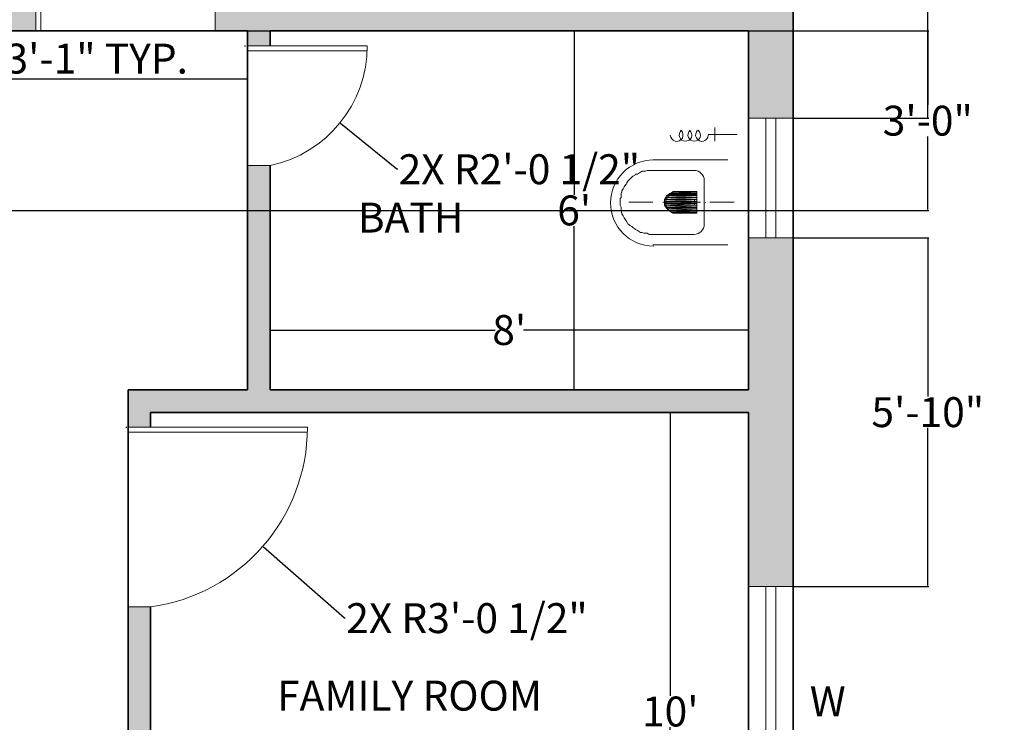
# Model space of a CAD drawing. Units: inches. Extents: x 302 to 1258, y 831 to 1373.
# Tile 5 of 13: x 569 to 767, y 1070 to 1211. Entities that reach past the tile are written whole.
import ezdxf

# ---------------------------------------------------------------- set-up
doc = ezdxf.new("R2010")
doc.units = ezdxf.units.IN
doc.header["$MEASUREMENT"] = 0
for name, color, linetype, lineweight in [('A-ANNO-DIMS', 2, 'Continuous', 18), ('A-ANNO-TEXT', 7, 'Continuous', 18), ('A-AREA-IDEN', 7, 'Continuous', 18), ('A-DOOR', 3, 'Continuous', 18), ('A-FLOR-FIXT', 8, 'Continuous', 18), ('A-GLAZ', 4, 'Continuous', 18), ('A-WALL', 7, 'Continuous', 35), ('A-WALL-PATT', 251, 'Continuous', 13)]:
    doc.layers.add(name, color=color, linetype=linetype, lineweight=lineweight)
doc.styles.get("Standard").update_dxf_attribs({"font": 'arial.ttf'})
doc.dimstyles.get("Standard").update_dxf_attribs({"dimtxt": 6, "dimasz": 0.18, "dimexe": 0.18, "dimexo": 0.0625, "dimgap": 0.09, "dimtad": 0, "dimtih": 1, "dimtoh": 1, "dimdec": 1, "dimzin": 0, "dimdsep": 46, "dimlunit": 3, "dimtxsty": 'Standard', "dimcen": 0.09, "dimadec": 0, "dimazin": 0, "dimtfac": 1, "dimtdec": 1, "dimtofl": 0, "dimtmove": 0, "dimatfit": 3, "dimfxl": 1, "dimtolj": 1, "dimtzin": 0, "dimarcsym": 0})

# ---------------------------------------------------------------- blocks, each defined once
blk = doc.blocks.new('*D9')
at = {"layer": 'A-ANNO-DIMS', "color": 0, "lineweight": -2, "transparency": 16777216}
for p, q in [((619.67, 1136.88), (619.67, 1149.01)), ((619.85, 1148.83), (664.82, 1148.83)), ((715.49, 1148.83), (670.52, 1148.83)), ((715.67, 1136.88), (715.67, 1149.01))]:
    blk.add_line(p, q, dxfattribs=at)
at = {"layer": 'A-ANNO-DIMS', "color": 0, "transparency": 16777216}
for points in [[(619.85, 1148.86), (619.85, 1148.8), (619.67, 1148.83)], [(715.49, 1148.86), (715.49, 1148.8), (715.67, 1148.83)]]:
    blk.add_solid(points, dxfattribs=at)
at = {"layer": 'Defpoints', "color": 0, "transparency": 16777216}
for p in [(715.67, 1148.83), (619.67, 1136.82), (715.67, 1136.82)]:
    blk.add_point(p, dxfattribs=at)
at = {"layer": 'A-ANNO-DIMS', "color": 0, "transparency": 16777216, "insert": (667.67, 1148.83), "char_height": 6, "attachment_point": 5}
blk.add_mtext("\\A1;8'", dxfattribs=at)
blk = doc.blocks.new('*D10')
at = {"layer": 'A-ANNO-DIMS', "color": 0, "lineweight": -2, "transparency": 16777216}
for p, q in [((715.61, 1208.82), (680.52, 1208.82)), ((680.7, 1208.64), (680.7, 1175.97)), ((680.7, 1137), (680.7, 1169.67)), ((715.61, 1136.82), (680.52, 1136.82))]:
    blk.add_line(p, q, dxfattribs=at)
at = {"layer": 'A-ANNO-DIMS', "color": 0, "transparency": 16777216}
for points in [[(680.67, 1208.64), (680.73, 1208.64), (680.7, 1208.82)], [(680.67, 1137), (680.73, 1137), (680.7, 1136.82)]]:
    blk.add_solid(points, dxfattribs=at)
at = {"layer": 'Defpoints', "color": 0, "transparency": 16777216}
for p in [(715.67, 1208.82), (680.7, 1136.82), (715.67, 1136.82)]:
    blk.add_point(p, dxfattribs=at)
at = {"layer": 'A-ANNO-DIMS', "color": 0, "transparency": 16777216, "insert": (680.7, 1172.82), "char_height": 6, "attachment_point": 5}
blk.add_mtext("\\A1;6'", dxfattribs=at)
blk = doc.blocks.new('*D12')
at = {"layer": 'A-ANNO-DIMS', "color": 0, "lineweight": -2, "transparency": 16777216}
for p, q in [((715.61, 1132.32), (699.81, 1132.32)), ((699.99, 1132.14), (699.99, 1075.47)), ((699.99, 1012.5), (699.99, 1069.17)), ((715.61, 1012.32), (699.81, 1012.32))]:
    blk.add_line(p, q, dxfattribs=at)
at = {"layer": 'A-ANNO-DIMS', "color": 0, "transparency": 16777216}
for points in [[(699.96, 1132.14), (700.02, 1132.14), (699.99, 1132.32)], [(699.96, 1012.5), (700.02, 1012.5), (699.99, 1012.32)]]:
    blk.add_solid(points, dxfattribs=at)
at = {"layer": 'Defpoints', "color": 0, "transparency": 16777216}
for p in [(715.67, 1132.32), (699.99, 1012.32), (715.67, 1012.32)]:
    blk.add_point(p, dxfattribs=at)
at = {"layer": 'A-ANNO-DIMS', "color": 0, "transparency": 16777216, "insert": (699.99, 1072.32), "char_height": 6, "attachment_point": 5}
blk.add_mtext("\\A1;10'", dxfattribs=at)
blk = doc.blocks.new('*D16')
at = {"layer": 'A-ANNO-DIMS', "color": 0, "lineweight": -2, "transparency": 16777216}
for p, q in [((459.17, 1208.76), (459.17, 1198.98)), ((615.17, 1208.76), (615.17, 1198.98)), ((459.35, 1199.16), (532.27, 1199.16)), ((614.99, 1199.16), (542.07, 1199.16))]:
    blk.add_line(p, q, dxfattribs=at)
at = {"layer": 'A-ANNO-DIMS', "color": 0, "transparency": 16777216}
for points in [[(459.35, 1199.19), (459.35, 1199.13), (459.17, 1199.16)], [(614.99, 1199.19), (614.99, 1199.13), (615.17, 1199.16)]]:
    blk.add_solid(points, dxfattribs=at)
at = {"layer": 'Defpoints', "color": 0, "transparency": 16777216}
for p in [(459.17, 1208.82), (615.17, 1208.82), (615.17, 1199.16)]:
    blk.add_point(p, dxfattribs=at)
at = {"layer": 'A-ANNO-DIMS', "color": 0, "transparency": 16777216, "insert": (537.17, 1199.16), "char_height": 6, "attachment_point": 5}
blk.add_mtext("\\A1;13'", dxfattribs=at)
blk = doc.blocks.new('WC-PLAN')
h = blk.add_hatch(color=256)
h.paths.add_polyline_path([(17.3, 10.16), (11.23, 10.16), (17.3, 9.71)])
h.paths.add_polyline_path([(11.23, 10.16), (17.3, 9.71), (11.08, 9.71)])
h = blk.add_hatch(color=256)
h.paths.add_polyline_path([(17.3, 10.32), (11.61, 10.32), (17.3, 10.16)])
h.paths.add_polyline_path([(11.61, 10.32), (17.3, 10.16), (11.23, 10.16)])
h = blk.add_hatch(color=256)
h.paths.add_polyline_path([(17.3, 10.54), (11.83, 10.54), (17.3, 10.32)])
h.paths.add_polyline_path([(11.83, 10.54), (17.3, 10.32), (11.61, 10.32)])
h = blk.add_hatch(color=256)
h.paths.add_polyline_path([(17.3, 10.7), (12.21, 10.7), (17.3, 10.54)])
h.paths.add_polyline_path([(12.21, 10.7), (17.3, 10.54), (11.83, 10.54)])
h = blk.add_hatch(color=256)
h.paths.add_polyline_path([(17.3, 10.92), (12.59, 10.92), (17.3, 10.7)])
h.paths.add_polyline_path([(12.59, 10.92), (17.3, 10.7), (12.21, 10.7)])
h = blk.add_hatch(color=256)
h.paths.add_polyline_path([(17.3, 9.71), (11.08, 9.71), (17.3, 9.33)])
h.paths.add_polyline_path([(11.08, 9.71), (17.3, 9.33), (10.85, 9.33)])
h = blk.add_hatch(color=256)
h.paths.add_polyline_path([(17.3, 9.33), (10.85, 9.33), (17.3, 8.95)])
h.paths.add_polyline_path([(10.85, 9.33), (17.3, 8.95), (10.85, 8.95)])
h = blk.add_hatch(color=256)
h.paths.add_polyline_path([(17.3, 8.95), (10.85, 8.95), (17.3, 8.57)])
h.paths.add_polyline_path([(10.85, 8.95), (17.3, 8.57), (10.85, 8.57)])
h = blk.add_hatch(color=256)
h.paths.add_polyline_path([(17.3, 8.57), (10.85, 8.57), (17.3, 8.19)])
h.paths.add_polyline_path([(10.85, 8.57), (17.3, 8.19), (10.85, 8.19)])
h = blk.add_hatch(color=256)
h.paths.add_polyline_path([(17.3, 8.19), (10.85, 8.19), (17.3, 7.81)])
h.paths.add_polyline_path([(10.85, 8.19), (17.3, 7.81), (11.08, 7.81)])
h = blk.add_hatch(color=256)
h.paths.add_polyline_path([(17.3, 7.81), (11.08, 7.81), (17.3, 7.59)])
h.paths.add_polyline_path([(11.08, 7.81), (17.3, 7.59), (11.23, 7.59)])
h = blk.add_hatch(color=256)
h.paths.add_polyline_path([(17.3, 7.59), (11.23, 7.59), (17.3, 7.21)])
h.paths.add_polyline_path([(11.23, 7.59), (17.3, 7.21), (11.61, 7.21)])
h = blk.add_hatch(color=256)
h.paths.add_polyline_path([(17.3, 7.21), (11.61, 7.21), (17.3, 7.05)])
h.paths.add_polyline_path([(11.61, 7.21), (17.3, 7.05), (11.83, 7.05)])
h = blk.add_hatch(color=256)
h.paths.add_polyline_path([(17.3, 7.05), (11.83, 7.05), (17.3, 6.83)])
h.paths.add_polyline_path([(11.83, 7.05), (17.3, 6.83), (12.21, 6.83)])
h = blk.add_hatch(color=256)
h.paths.add_polyline_path([(17.3, 6.83), (12.21, 6.83), (17.3, 6.6)])
h.paths.add_polyline_path([(12.21, 6.83), (17.3, 6.6), (12.59, 6.6)])
h.paths.add_polyline_path([(17.3, 6.6), (12.59, 6.6), (12.97, 6.6)])
for points in [[(20.94, 21.03), (20.94, 23.77), (20.94, 23.77)], [(25.41, 22.4), (19.57, 22.4), (19.57, 22.4)], [(23.52, 17.3), (8.5, 17.3), (8.5, 17.3)], [(9.48, 2.35), (8.72, 2.35), (8.12, 2.35), (7.74, 2.35), (7.36, 2.58), (6.98, 2.58), (6.75, 2.58), (6.37, 2.73), (5.99, 2.73), (5.61, 2.96), (5.39, 3.11), (5.01, 3.34), (4.85, 3.49), (4.48, 3.72), (4.25, 3.94), (3.87, 4.1), (3.64, 4.32), (3.49, 4.48), (3.26, 4.85), (3.11, 5.08), (2.88, 5.46), (2.73, 5.69), (2.5, 6.07), (2.28, 6.45), (2.28, 6.6), (2.12, 7.05), (2.12, 7.43), (2.12, 7.81), (1.9, 8.19), (1.9, 8.8), (1.9, 9.56), (2.12, 9.71), (2.12, 10.16), (2.12, 10.54), (2.28, 10.92), (2.28, 11.07), (2.5, 11.45), (2.73, 11.91), (2.88, 12.06), (3.11, 12.44), (3.26, 12.67), (3.49, 13.05), (3.64, 13.2), (3.87, 13.43), (4.25, 13.81), (4.48, 14.03), (4.85, 14.18), (5.01, 14.41), (5.39, 14.41), (5.61, 14.56), (5.99, 14.79), (6.37, 15.02), (6.75, 15.02), (6.98, 15.02), (7.36, 15.17), (7.74, 15.17), (8.12, 15.17), (8.72, 15.17), (9.48, 15.17)], [(16.69, 15.17), (9.48, 15.17), (9.48, 15.17)], [(18.81, 4.48), (18.81, 13.2), (18.81, 13.2)], [(17.3, 10.92), (12.97, 10.92), (12.97, 10.92)], [(17.3, 6.6), (17.3, 10.92), (17.3, 10.92)], [(8.5, 8.8), (3.64, 8.8), (3.64, 8.8)], [(18.05, 8.8), (10.47, 8.8), (10.47, 8.8)], [(16.84, 9.18), (16.92, 9.18), (16.92, 9.18)], [(16.84, 8.8), (16.84, 8.95), (16.84, 9.18)], [(16.84, 8.8), (16.92, 8.72), (16.92, 8.72)], [(16.84, 8.34), (16.84, 8.57), (16.84, 8.8)], [(16.84, 8.34), (16.92, 8.34), (16.92, 8.34)], [(19.04, 8.8), (19.04, 8.72), (19.04, 8.72)], [(24.81, 8.8), (19.95, 8.8), (19.95, 8.8)], [(17.3, 6.6), (12.97, 6.6), (12.97, 6.6)], [(16.69, 2.35), (9.48, 2.35), (9.48, 2.35)], [(23.52, 0.23), (8.5, 0.23), (8.5, 0.23)]]:
    blk.add_lwpolyline(points)
for points in [[(11.23, 10.16), (17.3, 9.71), (11.08, 9.71)], [(11.61, 10.32), (17.3, 10.16), (11.23, 10.16)], [(17.3, 10.16), (11.23, 10.16), (17.3, 9.71)], [(11.83, 10.54), (17.3, 10.32), (11.61, 10.32)], [(17.3, 10.32), (11.61, 10.32), (17.3, 10.16)], [(12.21, 10.7), (17.3, 10.54), (11.83, 10.54)], [(17.3, 10.54), (11.83, 10.54), (17.3, 10.32)], [(12.59, 10.92), (17.3, 10.7), (12.21, 10.7)], [(17.3, 10.7), (12.21, 10.7), (17.3, 10.54)], [(12.97, 10.92), (17.3, 10.92), (12.59, 10.92)], [(17.3, 10.92), (12.59, 10.92), (17.3, 10.7)], [(17.3, 10.92), (12.97, 10.92)], [(11.08, 9.71), (17.3, 9.33), (10.85, 9.33)], [(17.3, 9.33), (10.85, 9.33), (17.3, 8.95)], [(10.85, 9.33), (17.3, 8.95), (10.85, 8.95)], [(17.3, 8.95), (10.85, 8.95), (17.3, 8.57)], [(10.85, 8.95), (17.3, 8.57), (10.85, 8.57)], [(17.3, 8.57), (10.85, 8.57), (17.3, 8.19)], [(10.85, 8.57), (17.3, 8.19), (10.85, 8.19)], [(17.3, 8.19), (10.85, 8.19), (17.3, 7.81)], [(10.85, 8.19), (17.3, 7.81), (11.08, 7.81)], [(17.3, 9.71), (11.08, 9.71), (17.3, 9.33)], [(17.3, 7.81), (11.08, 7.81), (17.3, 7.59)], [(11.08, 7.81), (17.3, 7.59), (11.23, 7.59)], [(17.3, 7.59), (11.23, 7.59), (17.3, 7.21)], [(11.23, 7.59), (17.3, 7.21), (11.61, 7.21)], [(17.3, 7.21), (11.61, 7.21), (17.3, 7.05)], [(11.61, 7.21), (17.3, 7.05), (11.83, 7.05)], [(17.3, 7.05), (11.83, 7.05), (17.3, 6.83)], [(11.83, 7.05), (17.3, 6.83), (12.21, 6.83)], [(17.3, 6.83), (12.21, 6.83), (17.3, 6.6)], [(12.21, 6.83), (17.3, 6.6), (12.59, 6.6)], [(17.3, 6.6), (12.59, 6.6), (12.97, 6.6)], [(12.59, 6.6), (17.3, 6.6), (17.3, 6.6)]]:
    blk.add_lwpolyline(points, close=True)
for points, knots in [([(11.99, 22.25), (11.99, 21.72), (12.44, 21.19), (12.97, 21.03), (12.97, 21.03), (13.5, 20.88), (14.11, 21.19), (14.41, 21.64), (14.41, 21.64), (14.64, 22.17), (14.56, 22.78), (14.19, 23.16)], [0, 0, 0, 0, 0.083333, 0.083333, 0.083333, 0.083334, 0.166667, 0.166667, 0.166667, 0.166668, 1, 1, 1, 1]), ([(14.19, 23.23), (13.81, 22.86), (13.65, 22.32), (13.88, 21.79), (13.88, 21.79), (14.03, 21.34), (14.49, 21.03), (15.02, 21.03), (15.02, 21.03), (15.55, 21.03), (16.01, 21.34), (16.23, 21.79), (16.23, 21.79), (16.39, 22.32), (16.23, 22.86), (15.85, 23.23)], [0, 0, 0, 0, 0.0625, 0.0625, 0.0625, 0.062501, 0.125, 0.125, 0.125, 0.125001, 0.1875, 0.1875, 0.1875, 0.187501, 1, 1, 1, 1]), ([(15.93, 23.16), (15.55, 22.86), (15.4, 22.25), (15.63, 21.79), (15.63, 21.79), (15.78, 21.34), (16.31, 21.03), (16.76, 21.03), (16.76, 21.03), (17.3, 21.03), (17.75, 21.34), (17.98, 21.79), (17.98, 21.79), (18.13, 22.32), (17.98, 22.86), (17.6, 23.23)], [0, 0, 0, 0, 0.0625, 0.0625, 0.0625, 0.062501, 0.125, 0.125, 0.125, 0.125001, 0.1875, 0.1875, 0.1875, 0.187501, 1, 1, 1, 1]), ([(17.45, 23.23), (17.07, 22.86), (16.92, 22.17), (17.22, 21.72), (17.22, 21.72), (17.52, 21.19), (18.05, 20.88), (18.66, 21.03), (18.66, 21.03), (19.19, 21.19), (19.57, 21.72), (19.57, 22.25)], [0, 0, 0, 0, 0.083333, 0.083333, 0.083333, 0.083334, 0.166667, 0.166667, 0.166667, 0.166668, 1, 1, 1, 1]), ([(8.65, 17.3), (3.87, 17.3), (0, 13.43), (0, 8.65), (0, 8.65), (0, 3.87), (3.87, 0), (8.65, 0)], [0, 0, 0, 0, 0.125, 0.125, 0.125, 0.125001, 1, 1, 1, 1]), ([(13.12, 10.7), (11.99, 10.7), (11.08, 9.79), (11.08, 8.65), (11.08, 8.65), (11.08, 7.51), (11.99, 6.6), (13.12, 6.6)], [0, 0, 0, 0, 0.125, 0.125, 0.125, 0.125001, 1, 1, 1, 1])]:
    blk.add_open_spline(points, degree=3, knots=knots)
for points in [[(18.81, 13.12), (18.81, 14.26), (17.9, 15.17), (16.76, 15.17)], [(16.76, 2.35), (17.9, 2.35), (18.81, 3.26), (18.81, 4.4)]]:
    blk.add_open_spline(points, degree=3)
blk = doc.blocks.new('WINDOW-48IN')
for p, q in [((0, 0), (0, 9)), ((0, 9), (48, 9)), ((48, 9), (48, 0)), ((0, 5.5), (48, 5.5)), ((48, 3.5), (0, 3.5)), ((48, 0), (0, 0))]:
    blk.add_line(p, q)
blk = doc.blocks.new('VENT-WINDOW-24IN')
for p, q in [((0, 24), (9, 24)), ((0, 0), (0, 24)), ((3.5, 0), (3.5, 24)), ((5.5, 24), (5.5, 0)), ((9, 24), (9, 0)), ((9, 0), (0, 0))]:
    blk.add_line(p, q)
blk = doc.blocks.new('DOOR-36IN-BEDROOM')
for p, q in [((35, 36), (35, 0)), ((36, 0), (36, 36)), ((36, 36), (36, 0)), ((0, 0), (0, 4.5)), ((36, 0), (0, 0)), ((37, 0), (36, 0))]:
    blk.add_line(p, q)
blk.add_arc((36, -0.32), 36.32, 90, 172.3719)
blk = doc.blocks.new('DOOR-24IN-BATH')
for p, q in [((0, 27), (0, 24)), ((0, 24), (24, 24)), ((24, 24), (0, 24)), ((0, 24), (0, 0)), ((24, 23), (0, 23)), ((0, 0), (4.5, 0))]:
    blk.add_line(p, q)
blk.add_arc((-0.52, 24), 24.52, 281.8123, 0)
blk = doc.blocks.new('DOOR-36IN-ROOM')
for p, q in [((0, 39), (0, 36)), ((0, 36), (36, 36)), ((36, 36), (0, 36)), ((0, 36), (0, 0)), ((36, 35), (0, 35)), ((0, 0), (4.5, 0))]:
    blk.add_line(p, q)
blk.add_arc((-0.32, 36), 36.32, 277.6281, 0)
blk = doc.blocks.new('*D55')
at = {"layer": 'A-ANNO-DIMS', "color": 0, "lineweight": -2, "transparency": 16777216}
for p, q in [((459.67, 1208.76), (459.67, 1203.09)), ((496.67, 1208.76), (496.67, 1203.09)), ((459.85, 1203.27), (496.49, 1203.27)), ((496.67, 1203.27), (496.85, 1203.27))]:
    blk.add_line(p, q, dxfattribs=at)
at = {"layer": 'A-ANNO-DIMS', "color": 0, "transparency": 16777216}
for points in [[(459.85, 1203.3), (459.85, 1203.24), (459.67, 1203.27)], [(496.49, 1203.3), (496.49, 1203.24), (496.67, 1203.27)]]:
    blk.add_solid(points, dxfattribs=at)
at = {"layer": 'Defpoints', "color": 0, "transparency": 16777216}
for p in [(459.67, 1208.82), (496.67, 1208.82), (496.67, 1203.27)]:
    blk.add_point(p, dxfattribs=at)
at = {"layer": 'A-ANNO-DIMS', "color": 0, "transparency": 16777216, "insert": (551.65, 1203.27), "char_height": 6, "attachment_point": 5}
blk.add_mtext('\\A1;BEDROOM DOOR 3\'-1" TYP.', dxfattribs=at)
blk = doc.blocks.new('*D76')
at = {"layer": 'A-ANNO-DIMS', "color": 0, "lineweight": -2, "transparency": 16777216}
for p, q in [((724.73, 1254.71), (751.85, 1254.71)), ((751.67, 1254.53), (751.67, 1226.2)), ((751.67, 1191.48), (751.67, 1219.81)), ((724.73, 1191.3), (751.85, 1191.3))]:
    blk.add_line(p, q, dxfattribs=at)
at = {"layer": 'A-ANNO-DIMS', "color": 0, "transparency": 16777216}
for points in [[(751.64, 1254.53), (751.7, 1254.53), (751.67, 1254.71)], [(751.64, 1191.48), (751.7, 1191.48), (751.67, 1191.3)]]:
    blk.add_solid(points, dxfattribs=at)
at = {"layer": 'Defpoints', "color": 0, "transparency": 16777216}
for p in [(724.67, 1254.71), (724.67, 1191.3), (751.67, 1191.3)]:
    blk.add_point(p, dxfattribs=at)
at = {"layer": 'A-ANNO-DIMS', "color": 0, "transparency": 16777216, "insert": (751.67, 1223), "char_height": 6, "attachment_point": 5}
blk.add_mtext('\\A1;5\'-3 1/2"', dxfattribs=at)
blk = doc.blocks.new('*D77')
at = {"layer": 'A-ANNO-DIMS', "color": 0, "lineweight": -2, "transparency": 16777216}
for p, q in [((724.73, 1167.3), (751.85, 1167.3)), ((751.67, 1167.12), (751.67, 1135.51)), ((751.67, 1097.6), (751.67, 1129.21)), ((724.73, 1097.42), (751.85, 1097.42))]:
    blk.add_line(p, q, dxfattribs=at)
at = {"layer": 'A-ANNO-DIMS', "color": 0, "transparency": 16777216}
for points in [[(751.64, 1167.12), (751.7, 1167.12), (751.67, 1167.3)], [(751.64, 1097.6), (751.7, 1097.6), (751.67, 1097.42)]]:
    blk.add_solid(points, dxfattribs=at)
at = {"layer": 'Defpoints', "color": 0, "transparency": 16777216}
for p in [(724.67, 1167.3), (724.67, 1097.42), (751.67, 1097.42)]:
    blk.add_point(p, dxfattribs=at)
at = {"layer": 'A-ANNO-DIMS', "color": 0, "transparency": 16777216, "insert": (751.67, 1132.36), "char_height": 6, "attachment_point": 5}
blk.add_mtext('\\A1;5\'-10"', dxfattribs=at)
blk = doc.blocks.new('*D83')
at = {"layer": 'A-ANNO-DIMS', "color": 0, "lineweight": -2, "transparency": 16777216}
for p, q in [((376.73, 1208.82), (751.85, 1208.82)), ((751.67, 1208.64), (751.67, 1193.97)), ((751.67, 1173), (751.67, 1187.66)), ((376.73, 1172.82), (751.85, 1172.82))]:
    blk.add_line(p, q, dxfattribs=at)
at = {"layer": 'A-ANNO-DIMS', "color": 0, "transparency": 16777216}
for points in [[(751.64, 1208.64), (751.7, 1208.64), (751.67, 1208.82)], [(751.64, 1173), (751.7, 1173), (751.67, 1172.82)]]:
    blk.add_solid(points, dxfattribs=at)
at = {"layer": 'Defpoints', "color": 0, "transparency": 16777216}
for p in [(376.67, 1208.82), (751.67, 1208.82), (376.67, 1172.82)]:
    blk.add_point(p, dxfattribs=at)
at = {"layer": 'A-ANNO-DIMS', "color": 0, "transparency": 16777216, "insert": (751.67, 1190.82), "char_height": 6, "attachment_point": 5}
blk.add_mtext('\\A1;3\'-0"', dxfattribs=at)
blk = doc.blocks.new('*D94')
at = {"layer": 'A-ANNO-DIMS', "color": 0, "lineweight": -2, "transparency": 16777216}
for p, q in [((590.76, 1129.32), (590.94, 1129.32)), ((590.85, 1129.23), (590.85, 1129.41)), ((634.58, 1091.05), (618.32, 1105.28)), ((634.76, 1091.05), (634.58, 1091.05))]:
    blk.add_line(p, q, dxfattribs=at)
at = {"layer": 'A-ANNO-DIMS', "color": 0, "transparency": 16777216}
blk.add_solid([(618.34, 1105.3), (618.3, 1105.26), (618.18, 1105.4)], dxfattribs=at)
at = {"layer": 'Defpoints', "color": 0, "transparency": 16777216}
for p in [(590.85, 1129.32), (618.18, 1105.4)]:
    blk.add_point(p, dxfattribs=at)
at = {"layer": 'A-ANNO-DIMS', "color": 0, "transparency": 16777216, "insert": (659.19, 1091.05), "char_height": 6, "attachment_point": 5}
blk.add_mtext('\\A1;2X R3\'-0 1/2"', dxfattribs=at)
blk = doc.blocks.new('*D95')
at = {"layer": 'A-ANNO-DIMS', "color": 0, "lineweight": -2, "transparency": 16777216}
for p, q in [((614.56, 1205.82), (614.74, 1205.82)), ((614.65, 1205.73), (614.65, 1205.91)), ((645.1, 1181.08), (633.82, 1190.24)), ((645.28, 1181.08), (645.1, 1181.08))]:
    blk.add_line(p, q, dxfattribs=at)
at = {"layer": 'A-ANNO-DIMS', "color": 0, "transparency": 16777216}
blk.add_solid([(633.84, 1190.27), (633.8, 1190.22), (633.68, 1190.36)], dxfattribs=at)
at = {"layer": 'Defpoints', "color": 0, "transparency": 16777216}
for p in [(614.65, 1205.82), (633.68, 1190.36)]:
    blk.add_point(p, dxfattribs=at)
at = {"layer": 'A-ANNO-DIMS', "color": 0, "transparency": 16777216, "insert": (669.7, 1181.08), "char_height": 6, "attachment_point": 5}
blk.add_mtext('\\A1;2X R2\'-0 1/2"', dxfattribs=at)

msp = doc.modelspace()

# ---------------------------------------------------------------- hatches: boundary and pattern name
at = {"layer": 'A-WALL-PATT'}
h = msp.add_hatch(color=256, dxfattribs=at)
h.dxf.hatch_style = 1
h.paths.add_polyline_path([(524.78, 1342.32), (455.57, 1342.32), (455.57, 1333.32), (496.67, 1333.32), (496.67, 1330.32), (501.17, 1330.32), (501.17, 1333.32), (524.78, 1333.32)])
h.paths.add_polyline_path([(724.67, 1342.32), (548.78, 1342.32), (548.78, 1333.32), (567.17, 1333.32), (567.17, 1213.32), (501.17, 1213.32), (501.17, 1306.32), (496.67, 1306.32), (496.67, 1213.32), (495.67, 1213.32), (495.67, 1208.82), (496.67, 1208.82), (572.67, 1208.82), (572.67, 1213.32), (571.67, 1213.32), (571.67, 1333.32), (715.67, 1333.32), (715.67, 1302.71), (724.67, 1302.71)])
h.paths.add_polyline_path([(376.67, 1333.32), (407.57, 1333.32), (407.57, 1342.32), (367.67, 1342.32), (367.67, 1300.76), (376.67, 1300.76)])
h.paths.add_polyline_path([(459.67, 1213.32), (376.67, 1213.32), (376.67, 1252.76), (367.67, 1252.76), (367.67, 1164.55), (376.67, 1164.55), (376.67, 1208.82), (454.67, 1208.82), (454.67, 1082.82), (459.17, 1082.82), (459.17, 1208.82), (459.67, 1208.82)])
h.paths.add_polyline_path([(376.67, 1116.55), (367.67, 1116.55), (367.67, 1024.44), (376.67, 1024.44)])
h.paths.add_polyline_path([(724.67, 1254.71), (715.67, 1254.71), (715.67, 1213.32), (608.67, 1213.32), (608.67, 1208.82), (615.17, 1208.82), (615.17, 1205.82), (619.67, 1205.82), (619.67, 1208.82), (715.67, 1208.82), (715.67, 1191.3), (724.67, 1191.3)])
h.paths.add_polyline_path([(724.67, 1167.3), (715.67, 1167.3), (715.67, 1136.82), (619.67, 1136.82), (619.67, 1181.82), (615.17, 1181.82), (615.17, 1136.82), (591.17, 1136.82), (591.17, 1129.32), (595.67, 1129.32), (595.67, 1132.32), (715.67, 1132.32), (715.67, 1097.42), (724.67, 1097.42)])
h.paths.add_polyline_path([(724.67, 1049.42), (715.67, 1049.42), (715.67, 1012.32), (595.67, 1012.32), (595.67, 1093.32), (591.17, 1093.32), (591.17, 1007.82), (715.67, 1007.82), (715.67, 875.82), (709.67, 875.82), (709.67, 866.82), (715.67, 866.82), (724.67, 866.82)])
h.paths.add_polyline_path([(673.67, 875.82), (623.88, 875.82), (623.88, 866.82), (673.67, 866.82)], flags=17)
h.paths.add_polyline_path([(575.88, 875.82), (477.17, 875.82), (477.17, 971.82), (472.67, 971.82), (472.67, 875.82), (376.67, 875.82), (376.67, 896.2), (367.67, 896.2), (367.67, 866.82), (575.88, 866.82)])
h.paths.add_polyline_path([(376.67, 976.44), (367.67, 976.44), (367.67, 944.2), (376.67, 944.2)])

# ---------------------------------------------------------------- linework, layer by layer
at = {"layer": 'A-WALL'}
for p, q in [((724.67, 1342.32), (724.67, 866.82)), ((459.17, 1208.82), (615.17, 1208.82)), ((615.17, 1208.82), (615.17, 1136.82)), ((619.67, 1208.82), (619.67, 1205.82)), ((619.67, 1208.82), (715.67, 1208.82)), ((715.67, 1208.82), (715.67, 1136.82)), ((619.67, 1181.82), (619.67, 1136.82)), ((591.17, 1136.82), (591.17, 1007.82)), ((591.17, 1136.82), (615.17, 1136.82)), ((619.67, 1136.82), (715.67, 1136.82)), ((595.67, 1132.32), (595.67, 1129.32)), ((595.67, 1132.32), (715.67, 1132.32)), ((715.67, 1132.32), (715.67, 1012.32)), ((595.67, 1093.32), (595.67, 1012.32))]:
    msp.add_line(p, q, dxfattribs=at)

# ---------------------------------------------------------------- block references
at = {"layer": 'A-DOOR', "extrusion": (0, 0, -1), "zscale": -1}
msp.add_blockref('DOOR-36IN-BEDROOM', (-608.67, 1208.82), dxfattribs=at)
at = {"layer": 'A-DOOR'}
for name, p in [('DOOR-24IN-BATH', (615.17, 1181.82)), ('DOOR-36IN-ROOM', (591.17, 1093.32))]:
    msp.add_blockref(name, p, dxfattribs=at)
at = {"layer": 'A-FLOR-FIXT'}
msp.add_blockref('WC-PLAN', (688.01, 1165.67), dxfattribs=at)
at = {"layer": 'A-GLAZ'}
msp.add_blockref('VENT-WINDOW-24IN', (715.67, 1167.3), dxfattribs=at)
at = {"layer": 'A-GLAZ', "rotation": 269.9999999999995}
msp.add_blockref('WINDOW-48IN', (715.67, 1097.42), dxfattribs=at)

# ---------------------------------------------------------------- texts
at = {"layer": 'A-ANNO-TEXT', "insert": (728, 1077.36), "char_height": 6, "attachment_point": 1}
msp.add_mtext_dynamic_manual_height_columns('W', width=16.4894, gutter_width=30, heights=[0], dxfattribs=at)
at = {"layer": 'A-AREA-IDEN', "char_height": 6, "attachment_point": 1}
for s, width, insert in [('BATH', 36.3809, (637.28, 1174.38)), ('FAMILY ROOM', 61.3387, (621.08, 1078.5))]:
    msp.add_mtext_dynamic_manual_height_columns(s, width=width, gutter_width=30, heights=[0], dxfattribs=dict(at, insert=insert))

# ---------------------------------------------------------------- dimensions: what is measured, and where the dimension line sits
at = {"layer": 'A-ANNO-DIMS'}
for base, p1, p2, override, picture, middle in [((751.67, 1191.3), (724.67, 1254.71), (724.67, 1191.3), {"dimdec": 1, "dimlfac": 1, "dimrnd": 0, "dimzin": 1, "dimdsep": 46, "dimlunit": 4, "dimfrac": 2}, '*D76', (751.67, 1223)), ((751.67, 1208.82), (376.67, 1172.82), (376.67, 1208.82), {"dimdec": 1, "dimlfac": 1, "dimrnd": 0, "dimzin": 1, "dimdsep": 46, "dimlunit": 4, "dimfrac": 2}, '*D83', (751.67, 1190.82)), ((680.7, 1136.82), (715.67, 1208.82), (715.67, 1136.82), {"dimclrd": 0, "dimclre": 0, "dimclrt": 0}, '*D10', (680.7, 1172.82)), ((751.67, 1097.42), (724.67, 1167.3), (724.67, 1097.42), {"dimdec": 1, "dimlfac": 1, "dimrnd": 0, "dimzin": 1, "dimdsep": 46, "dimlunit": 4, "dimfrac": 2}, '*D77', (751.67, 1132.36)), ((699.99, 1012.32), (715.67, 1132.32), (715.67, 1012.32), {"dimclrd": 0, "dimclre": 0, "dimclrt": 0}, '*D12', (699.99, 1072.32))]:
    dim = msp.add_linear_dim(base=base, p1=p1, p2=p2, angle=90, dimstyle='Standard', override=override, dxfattribs=at)
    dim.commit()
    dim.dimension.update_dxf_attribs({"geometry": picture, "text_midpoint": middle})
dim = msp.add_linear_dim(base=(496.67, 1203.27), p1=(459.67, 1208.82), p2=(496.67, 1208.82), text='BEDROOM DOOR <> TYP.', dimstyle='Standard', override={"dimdec": 1, "dimlfac": 1, "dimrnd": 0, "dimzin": 1, "dimdsep": 46, "dimlunit": 4, "dimfrac": 2}, dxfattribs=at)
dim.commit()
dim.dimension.update_dxf_attribs({"geometry": '*D55', "text_midpoint": (551.65, 1203.27)})
for base, p1, p2, picture, middle in [((615.17, 1199.16), (459.17, 1208.82), (615.17, 1208.82), '*D16', (537.17, 1199.16)), ((715.67, 1148.83), (619.67, 1136.82), (715.67, 1136.82), '*D9', (667.67, 1148.83))]:
    dim = msp.add_linear_dim(base=base, p1=p1, p2=p2, dimstyle='Standard', override={"dimclrd": 0, "dimclre": 0, "dimclrt": 0}, dxfattribs=at)
    dim.commit()
    dim.dimension.update_dxf_attribs({"geometry": picture, "text_midpoint": middle})
for center, mpoint, picture, middle in [((614.65, 1205.82), (633.68, 1190.36), '*D95', (669.7, 1181.08)), ((590.85, 1129.32), (618.18, 1105.4), '*D94', (659.19, 1091.05))]:
    dim = msp.add_radius_dim(center=center, mpoint=mpoint, text='2X <>', dimstyle='Standard', override={"dimdec": 1, "dimlfac": 1, "dimrnd": 0, "dimzin": 1, "dimdsep": 46, "dimlunit": 4, "dimfrac": 2}, dxfattribs=at)
    dim.commit()
    dim.dimension.update_dxf_attribs({"geometry": picture, "text_midpoint": middle, "dimtype": 164})

doc.saveas('drawing.dxf')
